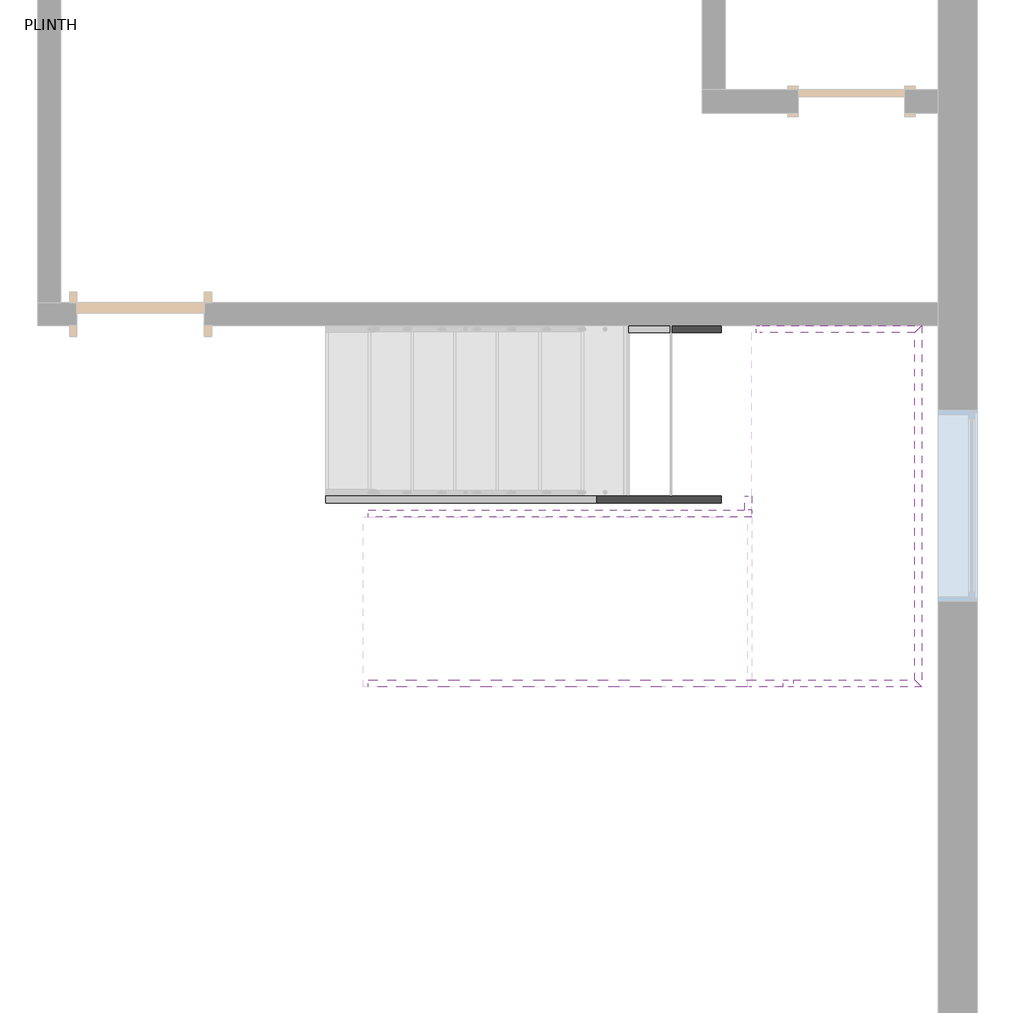
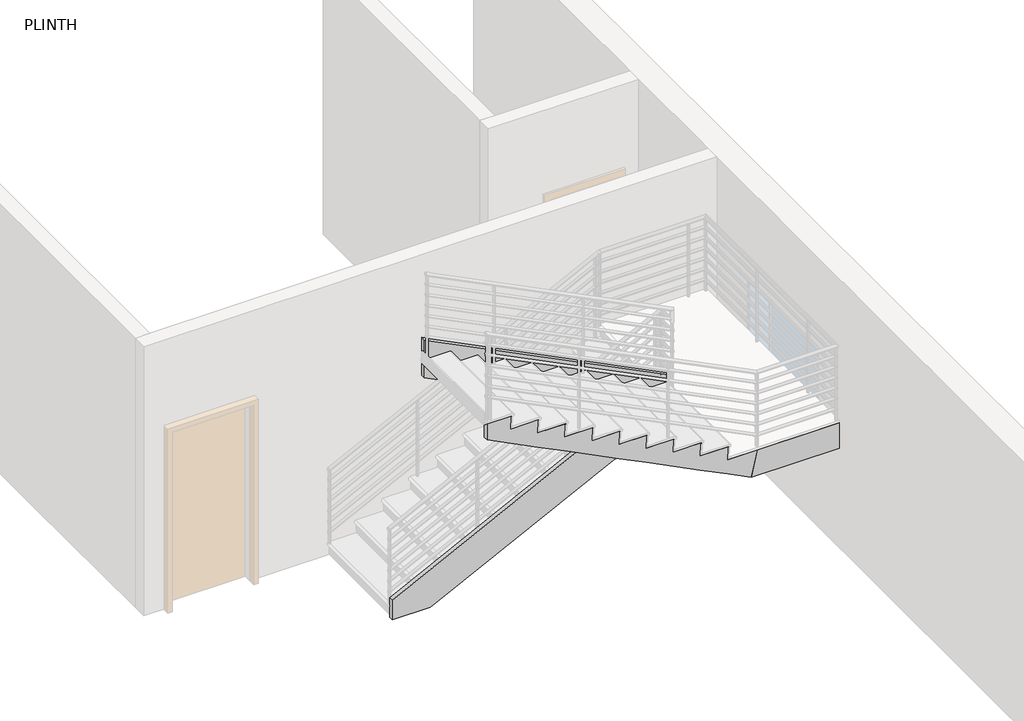
# One storey, part 4 of 4: 8 members.
"""IFC4 building model written with IfcOpenShell, lengths in millimetres."""

from ifc_helpers import new_model, si_unit, frame, origin, place, context, project, spatial, polyline, outline, extrude, faceted_brep, element, save

model = new_model("IFC4")

# Units and contexts
model_context = context("Model", 3, world=origin())
ifc_project = project(units=[si_unit("LENGTHUNIT", "METRE", prefix="MILLI")], contexts=[model_context])

# Site, building, storey
site = spatial("IfcSite", under=ifc_project)
building = spatial("IfcBuilding", under=site)
storey = spatial("IfcBuildingStorey", under=building, Name="PLINTH", Elevation=0.0)

# Members
placement = place(None, origin())
element("IfcMember", 1, ObjectType="Stringer - 50mm Width", at=placement, inside=storey, context=model_context, shape_type="Brep", body=[
    faceted_brep([(6886.9707523, 3626.4640673, 0.0), (7278.7829781, 3626.4640673, 0.0), (7278.7829781, 3576.4640673, 0.0), (6886.9707523, 3576.4640673, 0.0), (9935.1693537, 3626.4640673, 1519.5354413), (9975.570432, 3626.4640673, 1348.393727), (9936.1006455, 3626.4640673, 1328.6588337), (9897.4583908, 3626.4640673, 1309.3377063), (9631.3006455, 3626.4640673, 1176.2588337), (9326.5006455, 3626.4640673, 1023.8588337), (9021.7006455, 3626.4640673, 871.4588337), (8716.9006455, 3626.4640673, 719.0588337), (8412.1006455, 3626.4640673, 566.6588337), (8107.3006455, 3626.4640673, 414.2588337), (7802.5006455, 3626.4640673, 261.8588337), (7497.7006455, 3626.4640673, 109.4588337), (6881.3212861, 3626.4640673, 127.0), (7192.9006455, 3626.4640673, 127.0), (7186.1212861, 3626.4640673, 279.4), (7497.7006455, 3626.4640673, 279.4), (7490.9212861, 3626.4640673, 431.8), (7802.5006455, 3626.4640673, 431.8), (7795.7212861, 3626.4640673, 584.2), (8107.3006455, 3626.4640673, 584.2), (8100.5212861, 3626.4640673, 736.6), (8412.1006455, 3626.4640673, 736.6), (8405.3212861, 3626.4640673, 889.0), (8716.9006455, 3626.4640673, 889.0), (8710.1212861, 3626.4640673, 1041.4), (9021.7006455, 3626.4640673, 1041.4), (9014.9212861, 3626.4640673, 1193.8), (9326.5006455, 3626.4640673, 1193.8), (9319.7212861, 3626.4640673, 1346.2), (9631.3006455, 3626.4640673, 1346.2), (9624.5212861, 3626.4640673, 1498.6), (9897.4583908, 3626.4640673, 1498.6), (9936.1006455, 3626.4640673, 1498.6), (9975.570432, 3576.4640673, 1348.393727), (9935.1693537, 3576.4640673, 1519.5354413), (6881.3212861, 3576.4640673, 127.0), (7192.9006455, 3576.4640673, 127.0), (7186.1212861, 3576.4640673, 279.4), (7497.7006455, 3576.4640673, 279.4), (7490.9212861, 3576.4640673, 431.8), (7802.5006455, 3576.4640673, 431.8), (7795.7212861, 3576.4640673, 584.2), (8107.3006455, 3576.4640673, 584.2), (8100.5212861, 3576.4640673, 736.6), (8412.1006455, 3576.4640673, 736.6), (8405.3212861, 3576.4640673, 889.0), (8716.9006455, 3576.4640673, 889.0), (8710.1212861, 3576.4640673, 1041.4), (9021.7006455, 3576.4640673, 1041.4), (9014.9212861, 3576.4640673, 1193.8), (9326.5006455, 3576.4640673, 1193.8), (9319.7212861, 3576.4640673, 1346.2), (9631.3006455, 3576.4640673, 1346.2), (9624.5212861, 3576.4640673, 1498.6), (9936.1006455, 3576.4640673, 1498.6)], [[[0, 1, 2, 3]], [[4, 5, 6, 7, 8, 9, 10, 11, 12, 13, 14, 15, 1, 0, 16, 17, 18, 19, 20, 21, 22, 23, 24, 25, 26, 27, 28, 29, 30, 31, 32, 33, 34, 35, 36]], [[37, 5, 4, 38]], [[5, 37, 2, 1, 15, 14, 13, 12, 11, 10, 9, 8, 7, 6]], [[3, 39, 16, 0]], [[40, 17, 16, 39]], [[17, 40, 41, 18]], [[42, 19, 18, 41]], [[19, 42, 43, 20]], [[44, 21, 20, 43]], [[21, 44, 45, 22]], [[46, 23, 22, 45]], [[23, 46, 47, 24]], [[48, 25, 24, 47]], [[25, 48, 49, 26]], [[50, 27, 26, 49]], [[27, 50, 51, 28]], [[52, 29, 28, 51]], [[29, 52, 53, 30]], [[54, 31, 30, 53]], [[31, 54, 55, 32]], [[56, 33, 32, 55]], [[33, 56, 57, 34]], [[58, 36, 35, 34, 57]], [[36, 58, 38, 4]], [[2, 37, 38, 58, 57, 56, 55, 54, 53, 52, 51, 50, 49, 48, 47, 46, 45, 44, 43, 42, 41, 40, 39, 3]]]),
])
element("IfcMember", 2, ObjectType="Stringer - 50mm Width", at=placement, inside=storey, context=model_context, shape_type="SweptSolid", body=[
    extrude(outline(polyline([(232.5513018, 6849.4583908), (0.0, 6849.4583908), (0.0, 7278.7829781), (1284.3377063, 9847.4583908), (1731.5513018, 9847.4583908), (232.5513018, 6849.4583908)])), frame((0.0, 2357.2640673, 0.0), z_axis=(0.0, 1.0, 0.0), x_axis=(0.0, 0.0, 1.0)), (0.0, 0.0, 1.0), 50.0),
])
element("IfcMember", 3, ObjectType="Stringer - 50mm Width", at=placement, inside=storey, context=model_context, shape_type="Brep", body=[
    faceted_brep([(7154.2583908, 1088.0640673, 2833.3377063), (7154.2583908, 1038.0640673, 2833.3377063), (7154.2583908, 1038.0640673, 3022.6), (7154.2583908, 1088.0640673, 3022.6), (7420.416136, 1038.0640673, 2700.2588337), (7725.216136, 1038.0640673, 2547.8588337), (8030.016136, 1038.0640673, 2395.4588337), (8334.816136, 1038.0640673, 2243.0588337), (8639.616136, 1038.0640673, 2090.6588337), (8944.416136, 1038.0640673, 1938.2588337), (9249.216136, 1038.0640673, 1785.8588337), (9554.016136, 1038.0640673, 1633.4588337), (9858.816136, 1038.0640673, 1481.0588337), (9897.4583908, 1038.0640673, 1461.7377063), (10124.1463495, 1038.0640673, 1348.393727), (10195.5820003, 1038.0640673, 1651.0), (9897.4583908, 1038.0640673, 1651.0), (9858.816136, 1038.0640673, 1651.0), (9865.5954954, 1038.0640673, 1803.4), (9554.016136, 1038.0640673, 1803.4), (9560.7954954, 1038.0640673, 1955.8), (9249.216136, 1038.0640673, 1955.8), (9255.9954954, 1038.0640673, 2108.2), (8944.416136, 1038.0640673, 2108.2), (8951.1954954, 1038.0640673, 2260.6), (8639.616136, 1038.0640673, 2260.6), (8646.3954954, 1038.0640673, 2413.0), (8334.816136, 1038.0640673, 2413.0), (8341.5954954, 1038.0640673, 2565.4), (8030.016136, 1038.0640673, 2565.4), (8036.7954954, 1038.0640673, 2717.8), (7725.216136, 1038.0640673, 2717.8), (7731.9954954, 1038.0640673, 2870.2), (7420.416136, 1038.0640673, 2870.2), (7427.1954954, 1038.0640673, 3022.6), (10124.1463495, 1088.0640673, 1348.393727), (7427.1954954, 1088.0640673, 3022.6), (7420.416136, 1088.0640673, 2870.2), (7731.9954954, 1088.0640673, 2870.2), (7725.216136, 1088.0640673, 2717.8), (8036.7954954, 1088.0640673, 2717.8), (8030.016136, 1088.0640673, 2565.4), (8341.5954954, 1088.0640673, 2565.4), (8334.816136, 1088.0640673, 2413.0), (8646.3954954, 1088.0640673, 2413.0), (8639.616136, 1088.0640673, 2260.6), (8951.1954954, 1088.0640673, 2260.6), (8944.416136, 1088.0640673, 2108.2), (9255.9954954, 1088.0640673, 2108.2), (9249.216136, 1088.0640673, 1955.8), (9560.7954954, 1088.0640673, 1955.8), (9554.016136, 1088.0640673, 1803.4), (9865.5954954, 1088.0640673, 1803.4), (9858.816136, 1088.0640673, 1651.0), (10195.5820003, 1088.0640673, 1651.0)], [[[0, 1, 2, 3]], [[2, 1, 4, 5, 6, 7, 8, 9, 10, 11, 12, 13, 14, 15, 16, 17, 18, 19, 20, 21, 22, 23, 24, 25, 26, 27, 28, 29, 30, 31, 32, 33, 34]], [[1, 0, 35, 14, 13, 12, 11, 10, 9, 8, 7, 6, 5, 4]], [[35, 0, 3, 36, 37, 38, 39, 40, 41, 42, 43, 44, 45, 46, 47, 48, 49, 50, 51, 52, 53, 54]], [[14, 35, 54, 15]], [[51, 19, 18, 52]], [[52, 18, 17, 53]], [[49, 21, 20, 50]], [[19, 51, 50, 20]], [[47, 23, 22, 48]], [[21, 49, 48, 22]], [[45, 25, 24, 46]], [[23, 47, 46, 24]], [[43, 27, 26, 44]], [[25, 45, 44, 26]], [[41, 29, 28, 42]], [[27, 43, 42, 28]], [[39, 31, 30, 40]], [[29, 41, 40, 30]], [[37, 33, 32, 38]], [[31, 39, 38, 32]], [[34, 36, 3, 2]], [[33, 37, 36, 34]], [[53, 17, 16, 15, 54]]]),
])
element("IfcMember", 4, ObjectType="Stringer - 50mm Width", at=placement, inside=storey, context=model_context, shape_type="SweptSolid", body=[
    extrude(outline(polyline([(1461.7377063, 9897.4583908), (1908.9513018, 9897.4583908), (3280.5513018, 7154.2583908), (2833.3377063, 7154.2583908), (1461.7377063, 9897.4583908)])), frame((0.0, 2257.2640673, 0.0), z_axis=(0.0, 1.0, 0.0), x_axis=(0.0, 0.0, 1.0)), (0.0, 0.0, 1.0), 50.0),
])
element("IfcMember", 5, ObjectType="Stringer - 50mm Width", at=placement, inside=storey, context=model_context, shape_type="Brep", body=[
    faceted_brep([(11066.6583908, 1088.0640673, 1348.393727), (10124.1463495, 1088.0640673, 1348.393727), (10195.5820003, 1088.0640673, 1651.0), (11066.6583908, 1088.0640673, 1651.0), (11116.6583908, 1038.0640673, 1348.393727), (10124.1463495, 1038.0640673, 1348.393727), (11116.6583908, 1038.0640673, 1651.0), (10195.5820003, 1038.0640673, 1651.0)], [[[0, 1, 2, 3]], [[1, 0, 4, 5]], [[5, 4, 6, 7]], [[1, 5, 7, 2]], [[4, 0, 3, 6]], [[3, 2, 7, 6]]]),
])
element("IfcMember", 6, ObjectType="Stringer - 50mm Width", at=placement, inside=storey, context=model_context, shape_type="SweptSolid", body=[
    extrude(outline(polyline([(11066.6583908, 1088.0640673), (11066.6583908, 3576.4640673), (11116.6583908, 3626.4640673), (11116.6583908, 1038.0640673), (11066.6583908, 1088.0640673)])), frame((0.0, 0.0, 1348.393727), z_axis=(0.0, 0.0, 1.0), x_axis=(1.0, 0.0, 0.0)), (0.0, 0.0, 1.0), 302.606273),
])
element("IfcMember", 7, ObjectType="Stringer - 50mm Width", at=placement, inside=storey, context=model_context, shape_type="Brep", body=[
    faceted_brep([(9975.570432, 3576.4640673, 1348.393727), (11066.6583908, 3576.4640673, 1348.393727), (11066.6583908, 3576.4640673, 1651.0), (9929.3212861, 3576.4640673, 1651.0), (9935.1693537, 3576.4640673, 1519.5354413), (9975.570432, 3626.4640673, 1348.393727), (11116.6583908, 3626.4640673, 1348.393727), (9935.1693537, 3626.4640673, 1519.5354413), (9929.3212861, 3626.4640673, 1651.0), (11116.6583908, 3626.4640673, 1651.0)], [[[0, 1, 2, 3, 4]], [[1, 0, 5, 6]], [[6, 5, 7, 8, 9]], [[1, 6, 9, 2]], [[5, 0, 4, 7]], [[8, 3, 2, 9]], [[3, 8, 7, 4]]]),
])
element("IfcMember", 8, ObjectType="Stringer - 50mm Width", at=placement, inside=storey, context=model_context, shape_type="SweptSolid", body=[
    extrude(outline(polyline([(9847.4583908, 2407.2640673), (9897.4583908, 2407.2640673), (9897.4583908, 2307.2640673), (9847.4583908, 2307.2640673), (9847.4583908, 2407.2640673)])), frame((0.0, 0.0, 1348.393727), z_axis=(0.0, 0.0, 1.0), x_axis=(1.0, 0.0, 0.0)), (0.0, 0.0, 1.0), 400.0),
])

save(model, "model.ifc")

# Revit data of these elements
# Elements 1, 2, 3, 4, 5, 6, 7, 8 (IfcMember, "Stringer - 50mm Width")
#   Phase Created = New Construction
